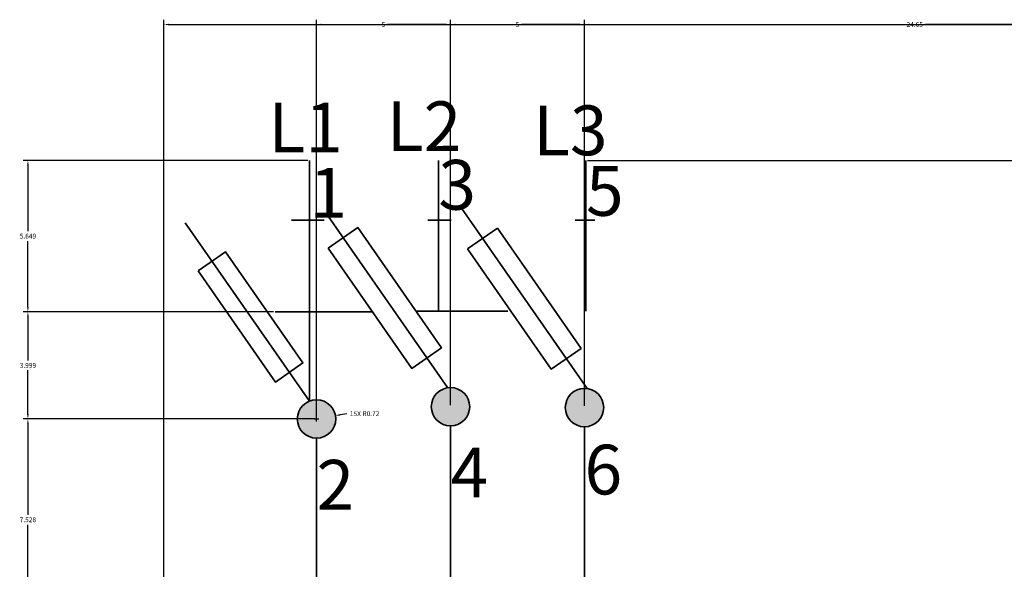
# Model space of a CAD drawing. Units: inches. Extents: x 237 to 313, y 343 to 451.
# Tile 4 of 6: x 237 to 274, y 431 to 451. Entities that reach past the tile are written whole.
import ezdxf

# ---------------------------------------------------------------- set-up
doc = ezdxf.new("R2010")
doc.units = ezdxf.units.IN
doc.header["$MEASUREMENT"] = 0
for name, color, linetype, lineweight in [('A-ANNO-DIMS', 2, 'Continuous', 18), ('E-ANNO-TEXT', 7, 'Continuous', 25), ('E-DEVC', 4, 'Continuous', 35), ('E-PATT', 8, 'Continuous', 13), ('E-WIRE', 7, 'Continuous', 35)]:
    doc.layers.add(name, color=color, linetype=linetype, lineweight=lineweight)
doc.styles.get("Standard").update_dxf_attribs({"font": 'arial.ttf'})
doc.dimstyles.get("Standard").update_dxf_attribs({"dimtxt": 0.18, "dimasz": 0.18, "dimexe": 0.18, "dimexo": 0.0625, "dimgap": 0.09, "dimtad": 0, "dimtih": 1, "dimtoh": 1, "dimdec": 4, "dimzin": 0, "dimdsep": 46, "dimtxsty": 'Standard', "dimcen": 0.09, "dimadec": 0, "dimazin": 0, "dimtfac": 1, "dimtdec": 4, "dimtofl": 0, "dimtmove": 0, "dimatfit": 3, "dimfxl": 1, "dimtolj": 1, "dimtzin": 0, "dimarcsym": 0})

# ---------------------------------------------------------------- blocks, each defined once
blk = doc.blocks.new('*D3')
at = {"layer": 'A-ANNO-DIMS', "color": 0, "lineweight": -2, "transparency": 16777216}
for p, q in [((242.3, 363.785), (242.3, 451.078)), ((242.48, 450.898), (274.084, 450.898)), ((306.476, 450.898), (274.872, 450.898)), ((306.656, 382.738), (306.656, 451.078))]:
    blk.add_line(p, q, dxfattribs=at)
at = {"layer": 'A-ANNO-DIMS', "color": 0, "lineweight": 35, "transparency": 16777216}
for points in [[(242.48, 450.928), (242.48, 450.868), (242.3, 450.898)], [(306.476, 450.928), (306.476, 450.868), (306.656, 450.898)]]:
    blk.add_solid(points, dxfattribs=at)
at = {"layer": 'Defpoints', "color": 0, "lineweight": 35, "transparency": 16777216}
for p in [(306.656, 450.898), (306.656, 382.675), (242.3, 363.723)]:
    blk.add_point(p, dxfattribs=at)
at = {"layer": 'A-ANNO-DIMS', "color": 0, "transparency": 16777216, "insert": (274.478, 450.898), "char_height": 0.18, "attachment_point": 5}
blk.add_mtext('\\A1;64.36', dxfattribs=at)
blk = doc.blocks.new('*D4')
at = {"layer": 'A-ANNO-DIMS', "color": 0, "lineweight": -2, "transparency": 16777216}
for p, q in [((258.115, 445.823), (312.65, 445.823)), ((312.47, 445.643), (312.47, 397.21)), ((312.47, 348.414), (312.47, 396.846)), ((289.124, 348.234), (312.65, 348.234))]:
    blk.add_line(p, q, dxfattribs=at)
at = {"layer": 'A-ANNO-DIMS', "color": 0, "lineweight": 35, "transparency": 16777216}
for points in [[(312.44, 445.643), (312.5, 445.643), (312.47, 445.823)], [(312.44, 348.414), (312.5, 348.414), (312.47, 348.234)]]:
    blk.add_solid(points, dxfattribs=at)
at = {"layer": 'Defpoints', "color": 0, "lineweight": 35, "transparency": 16777216}
for p in [(258.052, 445.823), (289.062, 348.234), (312.47, 348.234)]:
    blk.add_point(p, dxfattribs=at)
at = {"layer": 'A-ANNO-DIMS', "color": 0, "transparency": 16777216, "insert": (312.47, 397.028), "char_height": 0.18, "attachment_point": 5}
blk.add_mtext('\\A1;97.59', dxfattribs=at)
blk = doc.blocks.new('*D5')
at = {"layer": 'A-ANNO-DIMS', "color": 0, "lineweight": -2, "transparency": 16777216}
for p, q in [((247.997, 436.237), (247.997, 451.078)), ((248.177, 450.898), (250.347, 450.898)), ((252.817, 450.898), (250.647, 450.898)), ((252.997, 436.694), (252.997, 451.078))]:
    blk.add_line(p, q, dxfattribs=at)
at = {"layer": 'A-ANNO-DIMS', "color": 0, "lineweight": 35, "transparency": 16777216}
for points in [[(248.177, 450.928), (248.177, 450.868), (247.997, 450.898)], [(252.817, 450.928), (252.817, 450.868), (252.997, 450.898)]]:
    blk.add_solid(points, dxfattribs=at)
at = {"layer": 'Defpoints', "color": 0, "lineweight": 35, "transparency": 16777216}
for p in [(252.997, 450.898), (252.997, 436.631), (247.997, 436.174)]:
    blk.add_point(p, dxfattribs=at)
at = {"layer": 'A-ANNO-DIMS', "color": 0, "transparency": 16777216, "insert": (250.497, 450.898), "char_height": 0.18, "attachment_point": 5}
blk.add_mtext('\\A1;5', dxfattribs=at)
blk = doc.blocks.new('*D6')
at = {"layer": 'A-ANNO-DIMS', "color": 0, "lineweight": -2, "transparency": 16777216}
for p, q in [((252.997, 436.694), (252.997, 451.078)), ((253.177, 450.898), (255.347, 450.898)), ((257.817, 450.898), (255.647, 450.898)), ((257.997, 436.662), (257.997, 451.078))]:
    blk.add_line(p, q, dxfattribs=at)
at = {"layer": 'A-ANNO-DIMS', "color": 0, "lineweight": 35, "transparency": 16777216}
for points in [[(253.177, 450.928), (253.177, 450.868), (252.997, 450.898)], [(257.817, 450.928), (257.817, 450.868), (257.997, 450.898)]]:
    blk.add_solid(points, dxfattribs=at)
at = {"layer": 'Defpoints', "color": 0, "lineweight": 35, "transparency": 16777216}
for p in [(257.997, 450.898), (252.997, 436.631), (257.997, 436.599)]:
    blk.add_point(p, dxfattribs=at)
at = {"layer": 'A-ANNO-DIMS', "color": 0, "transparency": 16777216, "insert": (255.497, 450.898), "char_height": 0.18, "attachment_point": 5}
blk.add_mtext('\\A1;5', dxfattribs=at)
blk = doc.blocks.new('*D7')
at = {"layer": 'A-ANNO-DIMS', "color": 0, "lineweight": -2, "transparency": 16777216}
for p, q in [((257.997, 436.662), (257.997, 451.078)), ((258.177, 450.898), (269.926, 450.898)), ((282.468, 450.898), (270.718, 450.898)), ((282.648, 418.461), (282.648, 451.078))]:
    blk.add_line(p, q, dxfattribs=at)
at = {"layer": 'A-ANNO-DIMS', "color": 0, "lineweight": 35, "transparency": 16777216}
for points in [[(258.177, 450.928), (258.177, 450.868), (257.997, 450.898)], [(282.468, 450.928), (282.468, 450.868), (282.648, 450.898)]]:
    blk.add_solid(points, dxfattribs=at)
at = {"layer": 'Defpoints', "color": 0, "lineweight": 35, "transparency": 16777216}
for p in [(282.648, 450.898), (257.997, 436.599), (282.648, 418.399)]:
    blk.add_point(p, dxfattribs=at)
at = {"layer": 'A-ANNO-DIMS', "color": 0, "transparency": 16777216, "insert": (270.322, 450.898), "char_height": 0.18, "attachment_point": 5}
blk.add_mtext('\\A1;24.65', dxfattribs=at)
blk = doc.blocks.new('*D24')
at = {"layer": 'A-ANNO-DIMS', "color": 0, "lineweight": -2, "transparency": 16777216}
for p, q in [((247.667, 445.823), (237.045, 445.823)), ((237.225, 445.643), (237.225, 443.18)), ((237.225, 440.353), (237.225, 442.816)), ((246.389, 440.173), (237.045, 440.173))]:
    blk.add_line(p, q, dxfattribs=at)
at = {"layer": 'A-ANNO-DIMS', "color": 0, "lineweight": 35, "transparency": 16777216}
for points in [[(237.195, 445.643), (237.255, 445.643), (237.225, 445.823)], [(237.195, 440.353), (237.255, 440.353), (237.225, 440.173)]]:
    blk.add_solid(points, dxfattribs=at)
at = {"layer": 'Defpoints', "color": 0, "lineweight": 35, "transparency": 16777216}
for p in [(247.73, 445.823), (237.225, 440.173), (246.452, 440.173)]:
    blk.add_point(p, dxfattribs=at)
at = {"layer": 'A-ANNO-DIMS', "color": 0, "transparency": 16777216, "insert": (237.225, 442.998), "char_height": 0.18, "attachment_point": 5}
blk.add_mtext('\\A1;5.649', dxfattribs=at)
blk = doc.blocks.new('*D25')
at = {"layer": 'A-ANNO-DIMS', "color": 0, "lineweight": -2, "transparency": 16777216}
for p, q in [((246.389, 440.173), (237.045, 440.173)), ((237.225, 439.993), (237.225, 438.356)), ((237.225, 436.354), (237.225, 437.992)), ((247.934, 436.174), (237.045, 436.174))]:
    blk.add_line(p, q, dxfattribs=at)
at = {"layer": 'A-ANNO-DIMS', "color": 0, "lineweight": 35, "transparency": 16777216}
for points in [[(237.195, 439.993), (237.255, 439.993), (237.225, 440.173)], [(237.195, 436.354), (237.255, 436.354), (237.225, 436.174)]]:
    blk.add_solid(points, dxfattribs=at)
at = {"layer": 'Defpoints', "color": 0, "lineweight": 35, "transparency": 16777216}
for p in [(246.452, 440.173), (237.225, 436.174), (247.997, 436.174)]:
    blk.add_point(p, dxfattribs=at)
at = {"layer": 'A-ANNO-DIMS', "color": 0, "transparency": 16777216, "insert": (237.225, 438.174), "char_height": 0.18, "attachment_point": 5}
blk.add_mtext('\\A1;3.999', dxfattribs=at)
blk = doc.blocks.new('*D26')
at = {"layer": 'A-ANNO-DIMS', "color": 0, "lineweight": -2, "transparency": 16777216}
for p, q in [((247.934, 436.174), (237.045, 436.174)), ((237.225, 435.994), (237.225, 432.592)), ((237.225, 428.826), (237.225, 432.228)), ((257.943, 428.646), (237.045, 428.646))]:
    blk.add_line(p, q, dxfattribs=at)
at = {"layer": 'A-ANNO-DIMS', "color": 0, "lineweight": 35, "transparency": 16777216}
for points in [[(237.195, 435.994), (237.255, 435.994), (237.225, 436.174)], [(237.195, 428.826), (237.255, 428.826), (237.225, 428.646)]]:
    blk.add_solid(points, dxfattribs=at)
at = {"layer": 'Defpoints', "color": 0, "lineweight": 35, "transparency": 16777216}
for p in [(247.997, 436.174), (237.225, 428.646), (258.006, 428.646)]:
    blk.add_point(p, dxfattribs=at)
at = {"layer": 'A-ANNO-DIMS', "color": 0, "transparency": 16777216, "insert": (237.225, 432.41), "char_height": 0.18, "attachment_point": 5}
blk.add_mtext('\\A1;7.528', dxfattribs=at)
blk = doc.blocks.new('*D41')
at = {"layer": 'A-ANNO-DIMS', "color": 0, "lineweight": -2, "transparency": 16777216}
for p, q in [((247.997, 436.084), (247.997, 436.264)), ((249.127, 436.371), (248.88, 436.328)), ((247.907, 436.174), (248.087, 436.174))]:
    blk.add_line(p, q, dxfattribs=at)
at = {"layer": 'A-ANNO-DIMS', "color": 0, "lineweight": 35, "transparency": 16777216}
blk.add_solid([(248.875, 436.357), (248.886, 436.298), (248.703, 436.297)], dxfattribs=at)
at = {"layer": 'Defpoints', "color": 0, "lineweight": 35, "transparency": 16777216}
for p in [(248.703, 436.297), (247.997, 436.174)]:
    blk.add_point(p, dxfattribs=at)
at = {"layer": 'A-ANNO-DIMS', "color": 0, "transparency": 16777216, "insert": (249.791, 436.371), "char_height": 0.18, "attachment_point": 5}
blk.add_mtext('\\A1;15X R0.72', dxfattribs=at)

msp = doc.modelspace()

# ---------------------------------------------------------------- hatches: boundary and pattern name
at = {"layer": 'E-PATT'}
h = msp.add_hatch(color=256, dxfattribs=at)
h.dxf.hatch_style = 1
h.paths.add_polyline_path([(257.28, 436.5992, 1), (258.7137, 436.5992, 1)])
h.paths.add_polyline_path([(253.7137, 436.6313, 1), (252.28, 436.6313, 1)])
h.paths.add_polyline_path([(248.7137, 436.1741, 1), (247.28, 436.1741, 1)])

# ---------------------------------------------------------------- linework, layer by layer
at = {"layer": 'E-DEVC'}
for p, q in [((258.0963, 437.3091), (253.4124, 444.0415)), ((247.0672, 443.5891), (248.2849, 443.5891)), ((252.8837, 437.3435), (248.3421, 443.8713)), ((252.1537, 443.5891), (253.0182, 443.5891)), ((257.648, 443.5891), (258.3819, 443.5891)), ((247.7297, 436.8392), (243.097, 443.498)), ((246.4517, 440.1734), (250.1092, 440.1776)), ((251.7461, 440.1922), (255.1419, 440.1982))]:
    msp.add_line(p, q, dxfattribs=at)
for points in [[(248.4266, 442.5501), (249.5364, 443.3223), (252.66, 438.8326), (251.5502, 438.0604)], [(253.6345, 442.5225), (254.7443, 443.2946), (257.8679, 438.8049), (256.7581, 438.0328)], [(243.5785, 441.6975), (244.6039, 442.4109), (247.4897, 438.2629), (246.4643, 437.5495)]]:
    msp.add_lwpolyline(points, close=True, dxfattribs=at)
for centre in [(252.9968, 436.6313), (257.9968, 436.5992), (247.9968, 436.1741)]:
    msp.add_circle(centre, 0.7168, dxfattribs=at)
at = {"layer": 'E-WIRE'}
for p, q in [((247.7297, 436.8392), (247.7297, 445.8226)), ((252.5439, 440.1936), (252.5439, 445.8226)), ((258.0525, 440.1982), (258.0525, 445.8226)), ((252.9968, 435.9145), (252.9968, 418.3988)), ((257.9968, 435.8824), (257.9968, 418.3988)), ((247.9968, 435.4572), (247.9968, 416.8988))]:
    msp.add_line(p, q, dxfattribs=at)

# ---------------------------------------------------------------- texts
at = {"layer": 'E-ANNO-TEXT'}
for s, height, p in [('L1', 1.85645, (246.1984, 446.1264)), ('L2', 1.85645, (250.6163, 446.1699)), ('L3', 1.85645, (256.0789, 446.0177)), ('3', 1.8564, (252.5439, 443.9859)), ('1', 1.8564, (247.7297, 443.6874)), ('5', 1.8564, (258.0525, 443.7581)), ('4', 1.8564, (252.9968, 433.2424)), ('6', 1.8564, (257.9968, 433.3559)), ('2', 1.8564, (247.9968, 432.7883))]:
    msp.add_text(s, height=height, dxfattribs=at).set_placement(p)

# ---------------------------------------------------------------- dimensions: what is measured, and where the dimension line sits
at = {"layer": 'A-ANNO-DIMS'}
for base, p1, p2, override, picture, middle in [((306.6564, 450.8976), (242.3002, 363.7227), (306.6564, 382.675), {"dimdec": 2, "dimlfac": 1, "dimrnd": 0, "dimzin": 0, "dimdsep": 46, "dimlunit": 2}, '*D3', (274.4783, 450.8976)), ((252.9968, 450.8976), (247.9968, 436.1741), (252.9968, 436.6313), {"dimdec": 0, "dimlfac": 1, "dimrnd": 0, "dimzin": 0, "dimdsep": 46, "dimlunit": 2}, '*D5', (250.4968, 450.8976)), ((257.9968, 450.8976), (252.9968, 436.6313), (257.9968, 436.5992), {"dimdec": 0, "dimlfac": 1, "dimrnd": 0, "dimzin": 0, "dimdsep": 46, "dimlunit": 2}, '*D6', (255.4968, 450.8976)), ((282.6477, 450.8976), (257.9968, 436.5992), (282.6477, 418.3988), {"dimdec": 2, "dimlfac": 1, "dimrnd": 0, "dimzin": 0, "dimdsep": 46, "dimlunit": 2}, '*D7', (270.3223, 450.8976))]:
    dim = msp.add_linear_dim(base=base, p1=p1, p2=p2, dimstyle='Standard', override=override, dxfattribs=at)
    dim.commit()
    dim.dimension.update_dxf_attribs({"geometry": picture, "text_midpoint": middle})
for base, p1, p2, override, picture, middle in [((237.2252, 440.1734), (247.7297, 445.8226), (246.4517, 440.1734), {"dimdec": 3, "dimlfac": 1, "dimrnd": 0, "dimzin": 0, "dimdsep": 46, "dimlunit": 2}, '*D24', (237.2252, 442.998)), ((312.4701, 348.2337), (258.0525, 445.8226), (289.0615, 348.2337), {"dimdec": 2, "dimlfac": 1, "dimrnd": 0, "dimzin": 0, "dimdsep": 46, "dimlunit": 2}, '*D4', (312.4701, 397.0282)), ((237.2252, 436.1741), (246.4517, 440.1734), (247.9968, 436.1741), {"dimdec": 3, "dimlfac": 1, "dimrnd": 0, "dimzin": 0, "dimdsep": 46, "dimlunit": 2}, '*D25', (237.2252, 438.1737)), ((237.2252, 428.6459), (247.9968, 436.1741), (258.0057, 428.6459), {"dimdec": 3, "dimlfac": 1, "dimrnd": 0, "dimzin": 0, "dimdsep": 46, "dimlunit": 2}, '*D26', (237.2252, 432.41))]:
    dim = msp.add_linear_dim(base=base, p1=p1, p2=p2, angle=90, dimstyle='Standard', override=override, dxfattribs=at)
    dim.commit()
    dim.dimension.update_dxf_attribs({"geometry": picture, "text_midpoint": middle})
dim = msp.add_radius_dim(center=(247.9968, 436.1741), mpoint=(248.703, 436.297), text='15X <>', dimstyle='Standard', override={"dimdec": 2, "dimlfac": 1, "dimrnd": 0, "dimzin": 0, "dimdsep": 46, "dimlunit": 2}, dxfattribs=at)
dim.commit()
dim.dimension.update_dxf_attribs({"geometry": '*D41', "text_midpoint": (249.1268, 436.3708), "dimtype": 164})

doc.saveas('drawing.dxf')
